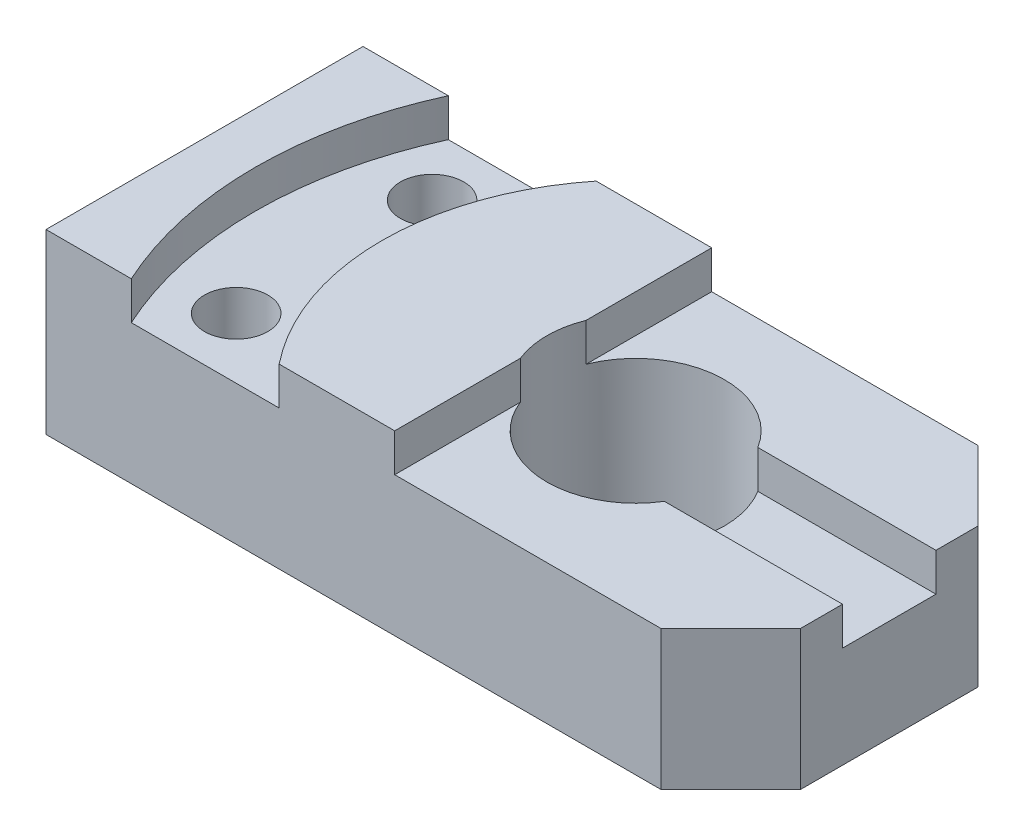
ISO-10303-21;
HEADER;
FILE_DESCRIPTION(('STEP AP214'),'2;1');
FILE_NAME('part.step','',(''),(''),'','','');
FILE_SCHEMA(('AUTOMOTIVE_DESIGN { 1 0 10303 214 1 1 1 1 }'));
ENDSEC;
DATA;
#1=APPLICATION_CONTEXT('core data for automotive mechanical design processes');
#2=APPLICATION_PROTOCOL_DEFINITION('international standard','automotive_design',2000,#1);
#3=PRODUCT_CONTEXT('',#1,'mechanical');
#4=PRODUCT('Part','Part','',(#3));
#5=PRODUCT_RELATED_PRODUCT_CATEGORY('part','',(#4));
#6=PRODUCT_DEFINITION_FORMATION('','',#4);
#7=PRODUCT_DEFINITION_CONTEXT('part definition',#1,'design');
#8=PRODUCT_DEFINITION('design','',#6,#7);
#9=PRODUCT_DEFINITION_SHAPE('','',#8);
#10=(LENGTH_UNIT() NAMED_UNIT(*) SI_UNIT(.MILLI.,.METRE.));
#11=(NAMED_UNIT(*) PLANE_ANGLE_UNIT() SI_UNIT($,.RADIAN.));
#12=(NAMED_UNIT(*) SI_UNIT($,.STERADIAN.) SOLID_ANGLE_UNIT());
#13=UNCERTAINTY_MEASURE_WITH_UNIT(LENGTH_MEASURE(1.E-05),#10,'distance_accuracy_value','');
#14=(GEOMETRIC_REPRESENTATION_CONTEXT(3) GLOBAL_UNCERTAINTY_ASSIGNED_CONTEXT((#13)) GLOBAL_UNIT_ASSIGNED_CONTEXT((#10,
#11,#12)) REPRESENTATION_CONTEXT('',''));
#15=CARTESIAN_POINT('',(0.,0.,0.));
#16=DIRECTION('',(0.,0.,1.));
#17=DIRECTION('',(1.,0.,0.));
#18=AXIS2_PLACEMENT_3D('',#15,#16,#17);
#19=CARTESIAN_POINT('',(0.,8.,0.));
#20=DIRECTION('',(0.,-1.,0.));
#21=DIRECTION('',(0.,0.,-1.));
#22=AXIS2_PLACEMENT_3D('',#19,#20,#21);
#23=PLANE('',#22);
#24=CARTESIAN_POINT('',(14.,8.,0.));
#25=DIRECTION('',(0.,-1.,0.));
#26=DIRECTION('',(0.,0.,-1.));
#27=AXIS2_PLACEMENT_3D('',#24,#25,#26);
#28=CIRCLE('',#27,14.);
#29=CARTESIAN_POINT('',(25.904726428639,8.,-7.36732574678661));
#30=VERTEX_POINT('',#29);
#31=CARTESIAN_POINT('',(0.99999999999999,8.,-5.19615242270663));
#32=VERTEX_POINT('',#31);
#33=EDGE_CURVE('E304',#30,#32,#28,.F.);
#34=ORIENTED_EDGE('',*,*,#33,.F.);
#35=DIRECTION('',(-1.,0.,0.));
#36=VECTOR('',#35,1.);
#37=CARTESIAN_POINT('',(25.904726428639,8.,-7.36732574678661));
#38=LINE('',#37,#36);
#39=CARTESIAN_POINT('',(54.,8.,-7.36732574678661));
#40=VERTEX_POINT('',#39);
#41=EDGE_CURVE('E185',#40,#30,#38,.T.);
#42=ORIENTED_EDGE('',*,*,#41,.F.);
#43=DIRECTION('',(0.,0.,-1.));
#44=VECTOR('',#43,1.);
#45=CARTESIAN_POINT('',(54.,8.,-13.9999999999999));
#46=LINE('',#45,#44);
#47=CARTESIAN_POINT('',(54.,8.,-13.9999999999999));
#48=VERTEX_POINT('',#47);
#49=EDGE_CURVE('E241',#40,#48,#46,.T.);
#50=ORIENTED_EDGE('',*,*,#49,.T.);
#51=DIRECTION('',(-0.707106781186546,0.,-0.707106781186549));
#52=VECTOR('',#51,1.);
#53=CARTESIAN_POINT('',(43.,8.,-25.));
#54=LINE('',#53,#52);
#55=CARTESIAN_POINT('',(43.,8.,-25.));
#56=VERTEX_POINT('',#55);
#57=EDGE_CURVE('E248',#48,#56,#54,.T.);
#58=ORIENTED_EDGE('',*,*,#57,.T.);
#59=DIRECTION('',(-1.,0.,0.));
#60=VECTOR('',#59,1.);
#61=CARTESIAN_POINT('',(0.999999999999987,8.,-25.));
#62=LINE('',#61,#60);
#63=CARTESIAN_POINT('',(0.999999999999987,8.,-25.));
#64=VERTEX_POINT('',#63);
#65=EDGE_CURVE('E234',#56,#64,#62,.T.);
#66=ORIENTED_EDGE('',*,*,#65,.T.);
#67=DIRECTION('',(0.,0.,1.));
#68=VECTOR('',#67,1.);
#69=CARTESIAN_POINT('',(0.999999999999987,8.,-25.));
#70=LINE('',#69,#68);
#71=EDGE_CURVE('E236',#64,#32,#70,.T.);
#72=ORIENTED_EDGE('',*,*,#71,.T.);
#73=EDGE_LOOP('',(#34,#42,#50,#58,#66,#72));
#74=FACE_BOUND('',#73,.T.);
#75=ADVANCED_FACE('F41',(#74),#23,.F.);
#76=CARTESIAN_POINT('',(0.,14.,0.));
#77=DIRECTION('',(0.,1.,0.));
#78=DIRECTION('',(0.,0.,1.));
#79=AXIS2_PLACEMENT_3D('',#76,#77,#78);
#80=PLANE('',#79);
#81=CARTESIAN_POINT('',(14.,14.,0.));
#82=DIRECTION('',(0.,-1.,0.));
#83=DIRECTION('',(0.,0.,1.));
#84=AXIS2_PLACEMENT_3D('',#81,#82,#83);
#85=CIRCLE('',#84,40.);
#86=CARTESIAN_POINT('',(-17.224989991992,14.,25.));
#87=VERTEX_POINT('',#86);
#88=CARTESIAN_POINT('',(-17.224989991992,14.,-25.));
#89=VERTEX_POINT('',#88);
#90=EDGE_CURVE('E203',#87,#89,#85,.T.);
#91=ORIENTED_EDGE('',*,*,#90,.F.);
#92=DIRECTION('',(1.,0.,0.));
#93=VECTOR('',#92,1.);
#94=CARTESIAN_POINT('',(-54.,14.,25.));
#95=LINE('',#94,#93);
#96=CARTESIAN_POINT('',(0.999999999999994,14.,25.));
#97=VERTEX_POINT('',#96);
#98=EDGE_CURVE('E269',#87,#97,#95,.T.);
#99=ORIENTED_EDGE('',*,*,#98,.T.);
#100=DIRECTION('',(0.,0.,1.));
#101=VECTOR('',#100,1.);
#102=CARTESIAN_POINT('',(0.999999999999987,14.,-25.));
#103=LINE('',#102,#101);
#104=CARTESIAN_POINT('',(0.999999999999991,14.,5.19615242270663));
#105=VERTEX_POINT('',#104);
#106=EDGE_CURVE('E228',#105,#97,#103,.T.);
#107=ORIENTED_EDGE('',*,*,#106,.F.);
#108=CARTESIAN_POINT('',(14.,14.,0.));
#109=DIRECTION('',(0.,1.,0.));
#110=DIRECTION('',(0.,0.,1.));
#111=AXIS2_PLACEMENT_3D('',#108,#109,#110);
#112=CIRCLE('',#111,14.);
#113=CARTESIAN_POINT('',(0.99999999999999,14.,-5.19615242270663));
#114=VERTEX_POINT('',#113);
#115=EDGE_CURVE('E258',#114,#105,#112,.T.);
#116=ORIENTED_EDGE('',*,*,#115,.F.);
#117=CARTESIAN_POINT('',(0.999999999999987,14.,-25.));
#118=VERTEX_POINT('',#117);
#119=EDGE_CURVE('E240',#118,#114,#103,.T.);
#120=ORIENTED_EDGE('',*,*,#119,.F.);
#121=DIRECTION('',(-1.,0.,0.));
#122=VECTOR('',#121,1.);
#123=CARTESIAN_POINT('',(-54.,14.,-25.));
#124=LINE('',#123,#122);
#125=EDGE_CURVE('E262',#118,#89,#124,.T.);
#126=ORIENTED_EDGE('',*,*,#125,.T.);
#127=EDGE_LOOP('',(#91,#99,#107,#116,#120,#126));
#128=FACE_BOUND('',#127,.T.);
#129=ADVANCED_FACE('F311',(#128),#80,.T.);
#130=CARTESIAN_POINT('',(54.,14.,-25.));
#131=DIRECTION('',(-1.,0.,0.));
#132=DIRECTION('',(0.,0.,1.));
#133=AXIS2_PLACEMENT_3D('',#130,#131,#132);
#134=PLANE('',#133);
#135=ORIENTED_EDGE('',*,*,#49,.F.);
#136=DIRECTION('',(0.,1.,0.));
#137=VECTOR('',#136,1.);
#138=CARTESIAN_POINT('',(54.,2.,-7.36732574678661));
#139=LINE('',#138,#137);
#140=CARTESIAN_POINT('',(54.,2.,-7.36732574678661));
#141=VERTEX_POINT('',#140);
#142=EDGE_CURVE('E190',#141,#40,#139,.T.);
#143=ORIENTED_EDGE('',*,*,#142,.F.);
#144=DIRECTION('',(0.,0.,-1.));
#145=VECTOR('',#144,1.);
#146=CARTESIAN_POINT('',(54.,2.,-7.36732574678661));
#147=LINE('',#146,#145);
#148=CARTESIAN_POINT('',(54.,2.,7.36732574678661));
#149=VERTEX_POINT('',#148);
#150=EDGE_CURVE('E174',#149,#141,#147,.T.);
#151=ORIENTED_EDGE('',*,*,#150,.F.);
#152=DIRECTION('',(0.,1.,0.));
#153=VECTOR('',#152,1.);
#154=CARTESIAN_POINT('',(54.,2.,7.36732574678661));
#155=LINE('',#154,#153);
#156=CARTESIAN_POINT('',(54.,8.,7.36732574678661));
#157=VERTEX_POINT('',#156);
#158=EDGE_CURVE('E166',#149,#157,#155,.T.);
#159=ORIENTED_EDGE('',*,*,#158,.T.);
#160=CARTESIAN_POINT('',(54.,8.,14.));
#161=VERTEX_POINT('',#160);
#162=EDGE_CURVE('E246',#161,#157,#46,.T.);
#163=ORIENTED_EDGE('',*,*,#162,.F.);
#164=DIRECTION('',(0.,-1.,0.));
#165=VECTOR('',#164,1.);
#166=CARTESIAN_POINT('',(54.,14.,14.));
#167=LINE('',#166,#165);
#168=CARTESIAN_POINT('',(54.,-14.,14.));
#169=VERTEX_POINT('',#168);
#170=EDGE_CURVE('E295',#161,#169,#167,.T.);
#171=ORIENTED_EDGE('',*,*,#170,.T.);
#172=DIRECTION('',(0.,0.,-1.));
#173=VECTOR('',#172,1.);
#174=CARTESIAN_POINT('',(54.,-14.,-25.));
#175=LINE('',#174,#173);
#176=CARTESIAN_POINT('',(54.,-14.,-13.9999999999999));
#177=VERTEX_POINT('',#176);
#178=EDGE_CURVE('E263',#169,#177,#175,.T.);
#179=ORIENTED_EDGE('',*,*,#178,.T.);
#180=DIRECTION('',(0.,1.,0.));
#181=VECTOR('',#180,1.);
#182=CARTESIAN_POINT('',(54.,14.,-13.9999999999999));
#183=LINE('',#182,#181);
#184=EDGE_CURVE('E288',#177,#48,#183,.T.);
#185=ORIENTED_EDGE('',*,*,#184,.T.);
#186=EDGE_LOOP('',(#135,#143,#151,#159,#163,#171,#179,#185));
#187=FACE_BOUND('',#186,.T.);
#188=ADVANCED_FACE('F339',(#187),#134,.F.);
#189=CARTESIAN_POINT('',(-54.,14.,-25.));
#190=DIRECTION('',(0.,0.,1.));
#191=DIRECTION('',(1.,0.,0.));
#192=AXIS2_PLACEMENT_3D('',#189,#190,#191);
#193=PLANE('',#192);
#194=DIRECTION('',(-1.,0.,0.));
#195=VECTOR('',#194,1.);
#196=CARTESIAN_POINT('',(-17.224989991992,8.,-25.));
#197=LINE('',#196,#195);
#198=CARTESIAN_POINT('',(-17.224989991992,8.,-25.));
#199=VERTEX_POINT('',#198);
#200=CARTESIAN_POINT('',(-40.5435605731786,8.,-25.));
#201=VERTEX_POINT('',#200);
#202=EDGE_CURVE('E211',#199,#201,#197,.T.);
#203=ORIENTED_EDGE('',*,*,#202,.F.);
#204=DIRECTION('',(0.,1.,0.));
#205=VECTOR('',#204,1.);
#206=CARTESIAN_POINT('',(-17.224989991992,8.,-25.));
#207=LINE('',#206,#205);
#208=EDGE_CURVE('E222',#199,#89,#207,.T.);
#209=ORIENTED_EDGE('',*,*,#208,.T.);
#210=ORIENTED_EDGE('',*,*,#125,.F.);
#211=DIRECTION('',(0.,1.,0.));
#212=VECTOR('',#211,1.);
#213=CARTESIAN_POINT('',(0.999999999999987,8.,-25.));
#214=LINE('',#213,#212);
#215=EDGE_CURVE('E253',#64,#118,#214,.T.);
#216=ORIENTED_EDGE('',*,*,#215,.F.);
#217=ORIENTED_EDGE('',*,*,#65,.F.);
#218=DIRECTION('',(0.,-1.,0.));
#219=VECTOR('',#218,1.);
#220=CARTESIAN_POINT('',(43.,14.,-25.));
#221=LINE('',#220,#219);
#222=CARTESIAN_POINT('',(43.,-14.,-25.));
#223=VERTEX_POINT('',#222);
#224=EDGE_CURVE('E301',#56,#223,#221,.T.);
#225=ORIENTED_EDGE('',*,*,#224,.T.);
#226=DIRECTION('',(-1.,0.,0.));
#227=VECTOR('',#226,1.);
#228=CARTESIAN_POINT('',(-54.,-14.,-25.));
#229=LINE('',#228,#227);
#230=CARTESIAN_POINT('',(-54.,-14.,-25.));
#231=VERTEX_POINT('',#230);
#232=EDGE_CURVE('E280',#223,#231,#229,.T.);
#233=ORIENTED_EDGE('',*,*,#232,.T.);
#234=DIRECTION('',(0.,-1.,0.));
#235=VECTOR('',#234,1.);
#236=CARTESIAN_POINT('',(-54.,14.,-25.));
#237=LINE('',#236,#235);
#238=CARTESIAN_POINT('',(-54.,14.,-25.));
#239=VERTEX_POINT('',#238);
#240=EDGE_CURVE('E286',#239,#231,#237,.T.);
#241=ORIENTED_EDGE('',*,*,#240,.F.);
#242=CARTESIAN_POINT('',(-40.5435605731786,14.,-25.));
#243=VERTEX_POINT('',#242);
#244=EDGE_CURVE('E268',#243,#239,#124,.T.);
#245=ORIENTED_EDGE('',*,*,#244,.F.);
#246=DIRECTION('',(0.,1.,0.));
#247=VECTOR('',#246,1.);
#248=CARTESIAN_POINT('',(-40.5435605731786,8.,-25.));
#249=LINE('',#248,#247);
#250=EDGE_CURVE('E61',#201,#243,#249,.T.);
#251=ORIENTED_EDGE('',*,*,#250,.F.);
#252=EDGE_LOOP('',(#203,#209,#210,#216,#217,#225,#233,#241,#245,#251));
#253=FACE_BOUND('',#252,.T.);
#254=ADVANCED_FACE('F359',(#253),#193,.F.);
#255=CARTESIAN_POINT('',(-54.,14.,-25.));
#256=DIRECTION('',(1.,0.,0.));
#257=DIRECTION('',(0.,0.,-1.));
#258=AXIS2_PLACEMENT_3D('',#255,#256,#257);
#259=PLANE('',#258);
#260=DIRECTION('',(0.,0.,1.));
#261=VECTOR('',#260,1.);
#262=CARTESIAN_POINT('',(-54.,-14.,-25.));
#263=LINE('',#262,#261);
#264=CARTESIAN_POINT('',(-54.,-14.,25.));
#265=VERTEX_POINT('',#264);
#266=EDGE_CURVE('E276',#231,#265,#263,.T.);
#267=ORIENTED_EDGE('',*,*,#266,.T.);
#268=DIRECTION('',(0.,-1.,0.));
#269=VECTOR('',#268,1.);
#270=CARTESIAN_POINT('',(-54.,14.,25.));
#271=LINE('',#270,#269);
#272=CARTESIAN_POINT('',(-54.,14.,25.));
#273=VERTEX_POINT('',#272);
#274=EDGE_CURVE('E273',#273,#265,#271,.T.);
#275=ORIENTED_EDGE('',*,*,#274,.F.);
#276=DIRECTION('',(0.,0.,1.));
#277=VECTOR('',#276,1.);
#278=CARTESIAN_POINT('',(-54.,14.,-25.));
#279=LINE('',#278,#277);
#280=EDGE_CURVE('E270',#239,#273,#279,.T.);
#281=ORIENTED_EDGE('',*,*,#280,.F.);
#282=ORIENTED_EDGE('',*,*,#240,.T.);
#283=EDGE_LOOP('',(#267,#275,#281,#282));
#284=FACE_BOUND('',#283,.T.);
#285=ADVANCED_FACE('F444',(#284),#259,.F.);
#286=CARTESIAN_POINT('',(-54.,14.,25.));
#287=DIRECTION('',(0.,0.,-1.));
#288=DIRECTION('',(-1.,0.,0.));
#289=AXIS2_PLACEMENT_3D('',#286,#287,#288);
#290=PLANE('',#289);
#291=ORIENTED_EDGE('',*,*,#98,.F.);
#292=DIRECTION('',(0.,1.,0.));
#293=VECTOR('',#292,1.);
#294=CARTESIAN_POINT('',(-17.224989991992,8.,25.));
#295=LINE('',#294,#293);
#296=CARTESIAN_POINT('',(-17.224989991992,8.,25.));
#297=VERTEX_POINT('',#296);
#298=EDGE_CURVE('E221',#297,#87,#295,.T.);
#299=ORIENTED_EDGE('',*,*,#298,.F.);
#300=DIRECTION('',(1.,0.,0.));
#301=VECTOR('',#300,1.);
#302=CARTESIAN_POINT('',(-40.5435605731786,8.,25.));
#303=LINE('',#302,#301);
#304=CARTESIAN_POINT('',(-40.5435605731786,8.,25.));
#305=VERTEX_POINT('',#304);
#306=EDGE_CURVE('E217',#305,#297,#303,.T.);
#307=ORIENTED_EDGE('',*,*,#306,.F.);
#308=DIRECTION('',(0.,1.,0.));
#309=VECTOR('',#308,1.);
#310=CARTESIAN_POINT('',(-40.5435605731786,8.,25.));
#311=LINE('',#310,#309);
#312=CARTESIAN_POINT('',(-40.5435605731786,14.,25.));
#313=VERTEX_POINT('',#312);
#314=EDGE_CURVE('E229',#305,#313,#311,.T.);
#315=ORIENTED_EDGE('',*,*,#314,.T.);
#316=EDGE_CURVE('E271',#273,#313,#95,.T.);
#317=ORIENTED_EDGE('',*,*,#316,.F.);
#318=ORIENTED_EDGE('',*,*,#274,.T.);
#319=DIRECTION('',(1.,0.,0.));
#320=VECTOR('',#319,1.);
#321=CARTESIAN_POINT('',(-54.,-14.,25.));
#322=LINE('',#321,#320);
#323=CARTESIAN_POINT('',(43.,-14.,25.));
#324=VERTEX_POINT('',#323);
#325=EDGE_CURVE('E283',#265,#324,#322,.T.);
#326=ORIENTED_EDGE('',*,*,#325,.T.);
#327=DIRECTION('',(0.,1.,0.));
#328=VECTOR('',#327,1.);
#329=CARTESIAN_POINT('',(43.,14.,25.));
#330=LINE('',#329,#328);
#331=CARTESIAN_POINT('',(43.,8.,25.));
#332=VERTEX_POINT('',#331);
#333=EDGE_CURVE('E297',#324,#332,#330,.T.);
#334=ORIENTED_EDGE('',*,*,#333,.T.);
#335=DIRECTION('',(1.,0.,0.));
#336=VECTOR('',#335,1.);
#337=CARTESIAN_POINT('',(43.,8.,25.));
#338=LINE('',#337,#336);
#339=CARTESIAN_POINT('',(0.999999999999994,8.,25.));
#340=VERTEX_POINT('',#339);
#341=EDGE_CURVE('E243',#340,#332,#338,.T.);
#342=ORIENTED_EDGE('',*,*,#341,.F.);
#343=DIRECTION('',(0.,1.,0.));
#344=VECTOR('',#343,1.);
#345=CARTESIAN_POINT('',(0.999999999999994,8.,25.));
#346=LINE('',#345,#344);
#347=EDGE_CURVE('E251',#340,#97,#346,.T.);
#348=ORIENTED_EDGE('',*,*,#347,.T.);
#349=EDGE_LOOP('',(#291,#299,#307,#315,#317,#318,#326,#334,#342,#348));
#350=FACE_BOUND('',#349,.T.);
#351=ADVANCED_FACE('F323',(#350),#290,.F.);
#352=CARTESIAN_POINT('',(14.,14.,0.));
#353=DIRECTION('',(0.,1.,0.));
#354=DIRECTION('',(0.,0.,1.));
#355=AXIS2_PLACEMENT_3D('',#352,#353,#354);
#356=CIRCLE('',#355,60.);
#357=EDGE_CURVE('E215',#243,#313,#356,.T.);
#358=ORIENTED_EDGE('',*,*,#357,.F.);
#359=ORIENTED_EDGE('',*,*,#244,.T.);
#360=ORIENTED_EDGE('',*,*,#280,.T.);
#361=ORIENTED_EDGE('',*,*,#316,.T.);
#362=EDGE_LOOP('',(#358,#359,#360,#361));
#363=FACE_BOUND('',#362,.T.);
#364=ADVANCED_FACE('F376',(#363),#80,.T.);
#365=CARTESIAN_POINT('',(0.,-14.,0.));
#366=DIRECTION('',(0.,1.,0.));
#367=DIRECTION('',(0.,0.,1.));
#368=AXIS2_PLACEMENT_3D('',#365,#366,#367);
#369=PLANE('',#368);
#370=CARTESIAN_POINT('',(-33.5528258147578,-14.,-15.4508497187471));
#371=DIRECTION('',(0.,1.,0.));
#372=DIRECTION('',(0.,0.,1.));
#373=AXIS2_PLACEMENT_3D('',#370,#371,#372);
#374=CIRCLE('',#373,5.);
#375=CARTESIAN_POINT('',(-33.5528258147578,-14.,-10.4508497187471));
#376=VERTEX_POINT('',#375);
#377=EDGE_CURVE('E197',#376,#376,#374,.F.);
#378=ORIENTED_EDGE('',*,*,#377,.F.);
#379=EDGE_LOOP('',(#378));
#380=FACE_BOUND('',#379,.T.);
#381=CARTESIAN_POINT('',(-33.5528258147578,-14.,15.4508497187471));
#382=DIRECTION('',(0.,1.,0.));
#383=DIRECTION('',(0.,0.,1.));
#384=AXIS2_PLACEMENT_3D('',#381,#382,#383);
#385=CIRCLE('',#384,5.);
#386=CARTESIAN_POINT('',(-33.5528258147578,-14.,20.4508497187471));
#387=VERTEX_POINT('',#386);
#388=EDGE_CURVE('E196',#387,#387,#385,.F.);
#389=ORIENTED_EDGE('',*,*,#388,.F.);
#390=EDGE_LOOP('',(#389));
#391=FACE_BOUND('',#390,.T.);
#392=CARTESIAN_POINT('',(14.,-14.,0.));
#393=DIRECTION('',(0.,1.,0.));
#394=DIRECTION('',(0.,0.,1.));
#395=AXIS2_PLACEMENT_3D('',#392,#393,#394);
#396=CIRCLE('',#395,14.);
#397=CARTESIAN_POINT('',(14.,-14.,14.));
#398=VERTEX_POINT('',#397);
#399=EDGE_CURVE('E257',#398,#398,#396,.F.);
#400=ORIENTED_EDGE('',*,*,#399,.F.);
#401=EDGE_LOOP('',(#400));
#402=FACE_BOUND('',#401,.T.);
#403=ORIENTED_EDGE('',*,*,#178,.F.);
#404=DIRECTION('',(0.707106781186549,0.,-0.707106781186547));
#405=VECTOR('',#404,1.);
#406=CARTESIAN_POINT('',(54.,-14.,14.));
#407=LINE('',#406,#405);
#408=EDGE_CURVE('E298',#169,#324,#407,.F.);
#409=ORIENTED_EDGE('',*,*,#408,.T.);
#410=ORIENTED_EDGE('',*,*,#325,.F.);
#411=ORIENTED_EDGE('',*,*,#266,.F.);
#412=ORIENTED_EDGE('',*,*,#232,.F.);
#413=DIRECTION('',(-0.707106781186546,0.,-0.707106781186549));
#414=VECTOR('',#413,1.);
#415=CARTESIAN_POINT('',(43.,-14.,-25.));
#416=LINE('',#415,#414);
#417=EDGE_CURVE('E294',#223,#177,#416,.F.);
#418=ORIENTED_EDGE('',*,*,#417,.T.);
#419=EDGE_LOOP('',(#403,#409,#410,#411,#412,#418));
#420=FACE_BOUND('',#419,.T.);
#421=ADVANCED_FACE('F470',(#380,#391,#402,#420),#369,.F.);
#422=CARTESIAN_POINT('',(54.,14.,14.));
#423=DIRECTION('',(-0.707106781186547,0.,-0.707106781186549));
#424=DIRECTION('',(0.,-1.,0.));
#425=AXIS2_PLACEMENT_3D('',#422,#423,#424);
#426=PLANE('',#425);
#427=DIRECTION('',(0.707106781186549,0.,-0.707106781186547));
#428=VECTOR('',#427,1.);
#429=CARTESIAN_POINT('',(54.,8.,14.));
#430=LINE('',#429,#428);
#431=EDGE_CURVE('E242',#332,#161,#430,.T.);
#432=ORIENTED_EDGE('',*,*,#431,.F.);
#433=ORIENTED_EDGE('',*,*,#333,.F.);
#434=ORIENTED_EDGE('',*,*,#408,.F.);
#435=ORIENTED_EDGE('',*,*,#170,.F.);
#436=EDGE_LOOP('',(#432,#433,#434,#435));
#437=FACE_BOUND('',#436,.T.);
#438=ADVANCED_FACE('F335',(#437),#426,.F.);
#439=CARTESIAN_POINT('',(43.,14.,-25.));
#440=DIRECTION('',(-0.707106781186549,0.,0.707106781186546));
#441=DIRECTION('',(0.,-1.,0.));
#442=AXIS2_PLACEMENT_3D('',#439,#440,#441);
#443=PLANE('',#442);
#444=ORIENTED_EDGE('',*,*,#57,.F.);
#445=ORIENTED_EDGE('',*,*,#184,.F.);
#446=ORIENTED_EDGE('',*,*,#417,.F.);
#447=ORIENTED_EDGE('',*,*,#224,.F.);
#448=EDGE_LOOP('',(#444,#445,#446,#447));
#449=FACE_BOUND('',#448,.T.);
#450=ADVANCED_FACE('F42',(#449),#443,.F.);
#451=CARTESIAN_POINT('',(14.,-53.5979797464467,0.));
#452=DIRECTION('',(0.,1.,0.));
#453=DIRECTION('',(0.,0.,1.));
#454=AXIS2_PLACEMENT_3D('',#451,#452,#453);
#455=CYLINDRICAL_SURFACE('',#454,14.);
#456=CARTESIAN_POINT('',(14.,2.,0.));
#457=DIRECTION('',(0.,-1.,0.));
#458=DIRECTION('',(0.,0.,1.));
#459=AXIS2_PLACEMENT_3D('',#456,#457,#458);
#460=CIRCLE('',#459,14.);
#461=CARTESIAN_POINT('',(25.904726428639,2.,-7.36732574678661));
#462=VERTEX_POINT('',#461);
#463=CARTESIAN_POINT('',(25.904726428639,2.,7.36732574678661));
#464=VERTEX_POINT('',#463);
#465=EDGE_CURVE('E172',#462,#464,#460,.T.);
#466=ORIENTED_EDGE('',*,*,#465,.F.);
#467=DIRECTION('',(0.,1.,0.));
#468=VECTOR('',#467,1.);
#469=CARTESIAN_POINT('',(25.904726428639,2.,-7.36732574678661));
#470=LINE('',#469,#468);
#471=EDGE_CURVE('E202',#462,#30,#470,.T.);
#472=ORIENTED_EDGE('',*,*,#471,.T.);
#473=ORIENTED_EDGE('',*,*,#33,.T.);
#474=DIRECTION('',(0.,1.,0.));
#475=VECTOR('',#474,1.);
#476=CARTESIAN_POINT('',(0.99999999999999,-53.5979797464467,-5.19615242270663));
#477=LINE('',#476,#475);
#478=EDGE_CURVE('E49',#32,#114,#477,.T.);
#479=ORIENTED_EDGE('',*,*,#478,.T.);
#480=ORIENTED_EDGE('',*,*,#115,.T.);
#481=DIRECTION('',(0.,1.,0.));
#482=VECTOR('',#481,1.);
#483=CARTESIAN_POINT('',(0.999999999999991,-53.5979797464467,5.19615242270663));
#484=LINE('',#483,#482);
#485=CARTESIAN_POINT('',(0.999999999999991,8.,5.19615242270663));
#486=VERTEX_POINT('',#485);
#487=EDGE_CURVE('E11',#105,#486,#484,.F.);
#488=ORIENTED_EDGE('',*,*,#487,.T.);
#489=CARTESIAN_POINT('',(25.904726428639,8.,7.36732574678661));
#490=VERTEX_POINT('',#489);
#491=EDGE_CURVE('E189',#486,#490,#28,.F.);
#492=ORIENTED_EDGE('',*,*,#491,.T.);
#493=DIRECTION('',(0.,1.,0.));
#494=VECTOR('',#493,1.);
#495=CARTESIAN_POINT('',(25.904726428639,2.,7.36732574678661));
#496=LINE('',#495,#494);
#497=EDGE_CURVE('E60',#464,#490,#496,.T.);
#498=ORIENTED_EDGE('',*,*,#497,.F.);
#499=EDGE_LOOP('',(#466,#472,#473,#479,#480,#488,#492,#498));
#500=FACE_BOUND('',#499,.T.);
#501=ORIENTED_EDGE('',*,*,#399,.T.);
#502=EDGE_LOOP('',(#501));
#503=FACE_BOUND('',#502,.T.);
#504=ADVANCED_FACE('F183',(#500,#503),#455,.F.);
#505=CARTESIAN_POINT('',(0.999999999999987,8.,-25.));
#506=DIRECTION('',(-1.,0.,0.));
#507=DIRECTION('',(0.,0.,1.));
#508=AXIS2_PLACEMENT_3D('',#505,#506,#507);
#509=PLANE('',#508);
#510=ORIENTED_EDGE('',*,*,#106,.T.);
#511=ORIENTED_EDGE('',*,*,#347,.F.);
#512=EDGE_CURVE('E237',#486,#340,#70,.T.);
#513=ORIENTED_EDGE('',*,*,#512,.F.);
#514=ORIENTED_EDGE('',*,*,#487,.F.);
#515=EDGE_LOOP('',(#510,#511,#513,#514));
#516=FACE_BOUND('',#515,.T.);
#517=ADVANCED_FACE('F317',(#516),#509,.F.);
#518=ORIENTED_EDGE('',*,*,#71,.F.);
#519=ORIENTED_EDGE('',*,*,#215,.T.);
#520=ORIENTED_EDGE('',*,*,#119,.T.);
#521=ORIENTED_EDGE('',*,*,#478,.F.);
#522=EDGE_LOOP('',(#518,#519,#520,#521));
#523=FACE_BOUND('',#522,.T.);
#524=ADVANCED_FACE('F358',(#523),#509,.F.);
#525=ORIENTED_EDGE('',*,*,#162,.T.);
#526=DIRECTION('',(1.,0.,0.));
#527=VECTOR('',#526,1.);
#528=CARTESIAN_POINT('',(25.904726428639,8.,7.36732574678661));
#529=LINE('',#528,#527);
#530=EDGE_CURVE('E340',#490,#157,#529,.T.);
#531=ORIENTED_EDGE('',*,*,#530,.F.);
#532=ORIENTED_EDGE('',*,*,#491,.F.);
#533=ORIENTED_EDGE('',*,*,#512,.T.);
#534=ORIENTED_EDGE('',*,*,#341,.T.);
#535=ORIENTED_EDGE('',*,*,#431,.T.);
#536=EDGE_LOOP('',(#525,#531,#532,#533,#534,#535));
#537=FACE_BOUND('',#536,.T.);
#538=ADVANCED_FACE('F327',(#537),#23,.F.);
#539=CARTESIAN_POINT('',(14.,8.,0.));
#540=DIRECTION('',(0.,1.,0.));
#541=DIRECTION('',(0.,0.,1.));
#542=AXIS2_PLACEMENT_3D('',#539,#540,#541);
#543=CYLINDRICAL_SURFACE('',#542,40.);
#544=ORIENTED_EDGE('',*,*,#90,.T.);
#545=ORIENTED_EDGE('',*,*,#208,.F.);
#546=CARTESIAN_POINT('',(14.,8.,0.));
#547=DIRECTION('',(0.,-1.,0.));
#548=DIRECTION('',(0.,0.,1.));
#549=AXIS2_PLACEMENT_3D('',#546,#547,#548);
#550=CIRCLE('',#549,40.);
#551=EDGE_CURVE('E208',#297,#199,#550,.T.);
#552=ORIENTED_EDGE('',*,*,#551,.F.);
#553=ORIENTED_EDGE('',*,*,#298,.T.);
#554=EDGE_LOOP('',(#544,#545,#552,#553));
#555=FACE_BOUND('',#554,.T.);
#556=ADVANCED_FACE('F370',(#555),#543,.T.);
#557=CARTESIAN_POINT('',(14.,8.,0.));
#558=DIRECTION('',(0.,1.,0.));
#559=DIRECTION('',(0.,0.,1.));
#560=AXIS2_PLACEMENT_3D('',#557,#558,#559);
#561=CYLINDRICAL_SURFACE('',#560,60.);
#562=ORIENTED_EDGE('',*,*,#357,.T.);
#563=ORIENTED_EDGE('',*,*,#314,.F.);
#564=CARTESIAN_POINT('',(14.,8.,0.));
#565=DIRECTION('',(0.,1.,0.));
#566=DIRECTION('',(0.,0.,1.));
#567=AXIS2_PLACEMENT_3D('',#564,#565,#566);
#568=CIRCLE('',#567,60.);
#569=EDGE_CURVE('E214',#201,#305,#568,.T.);
#570=ORIENTED_EDGE('',*,*,#569,.F.);
#571=ORIENTED_EDGE('',*,*,#250,.T.);
#572=EDGE_LOOP('',(#562,#563,#570,#571));
#573=FACE_BOUND('',#572,.T.);
#574=ADVANCED_FACE('F379',(#573),#561,.F.);
#575=CARTESIAN_POINT('',(14.,8.,0.));
#576=DIRECTION('',(0.,1.,0.));
#577=DIRECTION('',(0.,0.,1.));
#578=AXIS2_PLACEMENT_3D('',#575,#576,#577);
#579=PLANE('',#578);
#580=CARTESIAN_POINT('',(-33.5528258147578,8.,-15.4508497187471));
#581=DIRECTION('',(0.,1.,0.));
#582=DIRECTION('',(0.,0.,1.));
#583=AXIS2_PLACEMENT_3D('',#580,#581,#582);
#584=CIRCLE('',#583,5.);
#585=CARTESIAN_POINT('',(-33.5528258147578,8.,-10.4508497187471));
#586=VERTEX_POINT('',#585);
#587=EDGE_CURVE('E193',#586,#586,#584,.T.);
#588=ORIENTED_EDGE('',*,*,#587,.F.);
#589=EDGE_LOOP('',(#588));
#590=FACE_BOUND('',#589,.T.);
#591=CARTESIAN_POINT('',(-33.5528258147578,8.,15.4508497187471));
#592=DIRECTION('',(0.,1.,0.));
#593=DIRECTION('',(0.,0.,1.));
#594=AXIS2_PLACEMENT_3D('',#591,#592,#593);
#595=CIRCLE('',#594,5.);
#596=CARTESIAN_POINT('',(-33.5528258147578,8.,20.4508497187471));
#597=VERTEX_POINT('',#596);
#598=EDGE_CURVE('E205',#597,#597,#595,.T.);
#599=ORIENTED_EDGE('',*,*,#598,.F.);
#600=EDGE_LOOP('',(#599));
#601=FACE_BOUND('',#600,.T.);
#602=ORIENTED_EDGE('',*,*,#551,.T.);
#603=ORIENTED_EDGE('',*,*,#202,.T.);
#604=ORIENTED_EDGE('',*,*,#569,.T.);
#605=ORIENTED_EDGE('',*,*,#306,.T.);
#606=EDGE_LOOP('',(#602,#603,#604,#605));
#607=FACE_BOUND('',#606,.T.);
#608=ADVANCED_FACE('F383',(#590,#601,#607),#579,.T.);
#609=CARTESIAN_POINT('',(-33.5528258147578,-28.142135623731,15.4508497187471));
#610=DIRECTION('',(0.,1.,0.));
#611=DIRECTION('',(0.,0.,1.));
#612=AXIS2_PLACEMENT_3D('',#609,#610,#611);
#613=CYLINDRICAL_SURFACE('',#612,5.);
#614=ORIENTED_EDGE('',*,*,#388,.T.);
#615=EDGE_LOOP('',(#614));
#616=FACE_BOUND('',#615,.T.);
#617=ORIENTED_EDGE('',*,*,#598,.T.);
#618=EDGE_LOOP('',(#617));
#619=FACE_BOUND('',#618,.T.);
#620=ADVANCED_FACE('F390',(#616,#619),#613,.F.);
#621=CARTESIAN_POINT('',(-33.5528258147578,-28.142135623731,-15.4508497187471));
#622=DIRECTION('',(0.,1.,0.));
#623=DIRECTION('',(0.,0.,1.));
#624=AXIS2_PLACEMENT_3D('',#621,#622,#623);
#625=CYLINDRICAL_SURFACE('',#624,5.);
#626=ORIENTED_EDGE('',*,*,#377,.T.);
#627=EDGE_LOOP('',(#626));
#628=FACE_BOUND('',#627,.T.);
#629=ORIENTED_EDGE('',*,*,#587,.T.);
#630=EDGE_LOOP('',(#629));
#631=FACE_BOUND('',#630,.T.);
#632=ADVANCED_FACE('F393',(#628,#631),#625,.F.);
#633=CARTESIAN_POINT('',(25.904726428639,2.,-7.36732574678661));
#634=DIRECTION('',(0.,0.,-1.));
#635=DIRECTION('',(-1.,0.,0.));
#636=AXIS2_PLACEMENT_3D('',#633,#634,#635);
#637=PLANE('',#636);
#638=ORIENTED_EDGE('',*,*,#41,.T.);
#639=ORIENTED_EDGE('',*,*,#471,.F.);
#640=DIRECTION('',(-1.,0.,0.));
#641=VECTOR('',#640,1.);
#642=CARTESIAN_POINT('',(25.904726428639,2.,-7.36732574678661));
#643=LINE('',#642,#641);
#644=EDGE_CURVE('E178',#141,#462,#643,.T.);
#645=ORIENTED_EDGE('',*,*,#644,.F.);
#646=ORIENTED_EDGE('',*,*,#142,.T.);
#647=EDGE_LOOP('',(#638,#639,#645,#646));
#648=FACE_BOUND('',#647,.T.);
#649=ADVANCED_FACE('F350',(#648),#637,.F.);
#650=CARTESIAN_POINT('',(25.904726428639,2.,7.36732574678661));
#651=DIRECTION('',(0.,0.,1.));
#652=DIRECTION('',(1.,0.,0.));
#653=AXIS2_PLACEMENT_3D('',#650,#651,#652);
#654=PLANE('',#653);
#655=ORIENTED_EDGE('',*,*,#530,.T.);
#656=ORIENTED_EDGE('',*,*,#158,.F.);
#657=DIRECTION('',(1.,0.,0.));
#658=VECTOR('',#657,1.);
#659=CARTESIAN_POINT('',(25.904726428639,2.,7.36732574678661));
#660=LINE('',#659,#658);
#661=EDGE_CURVE('E164',#464,#149,#660,.T.);
#662=ORIENTED_EDGE('',*,*,#661,.F.);
#663=ORIENTED_EDGE('',*,*,#497,.T.);
#664=EDGE_LOOP('',(#655,#656,#662,#663));
#665=FACE_BOUND('',#664,.T.);
#666=ADVANCED_FACE('F170',(#665),#654,.F.);
#667=CARTESIAN_POINT('',(14.,2.,0.));
#668=DIRECTION('',(0.,1.,0.));
#669=DIRECTION('',(0.,0.,1.));
#670=AXIS2_PLACEMENT_3D('',#667,#668,#669);
#671=PLANE('',#670);
#672=ORIENTED_EDGE('',*,*,#465,.T.);
#673=ORIENTED_EDGE('',*,*,#661,.T.);
#674=ORIENTED_EDGE('',*,*,#150,.T.);
#675=ORIENTED_EDGE('',*,*,#644,.T.);
#676=EDGE_LOOP('',(#672,#673,#674,#675));
#677=FACE_BOUND('',#676,.T.);
#678=ADVANCED_FACE('F177',(#677),#671,.T.);
#679=CLOSED_SHELL('',(#75,#129,#188,#254,#285,#351,#364,#421,#438,#450,#504,#517,#524,#538,#556,
#574,#608,#620,#632,#649,#666,#678));
#680=MANIFOLD_SOLID_BREP('B2',#679);
#681=ADVANCED_BREP_SHAPE_REPRESENTATION('',(#18,#680),#14);
#682=SHAPE_DEFINITION_REPRESENTATION(#9,#681);
ENDSEC;
END-ISO-10303-21;
